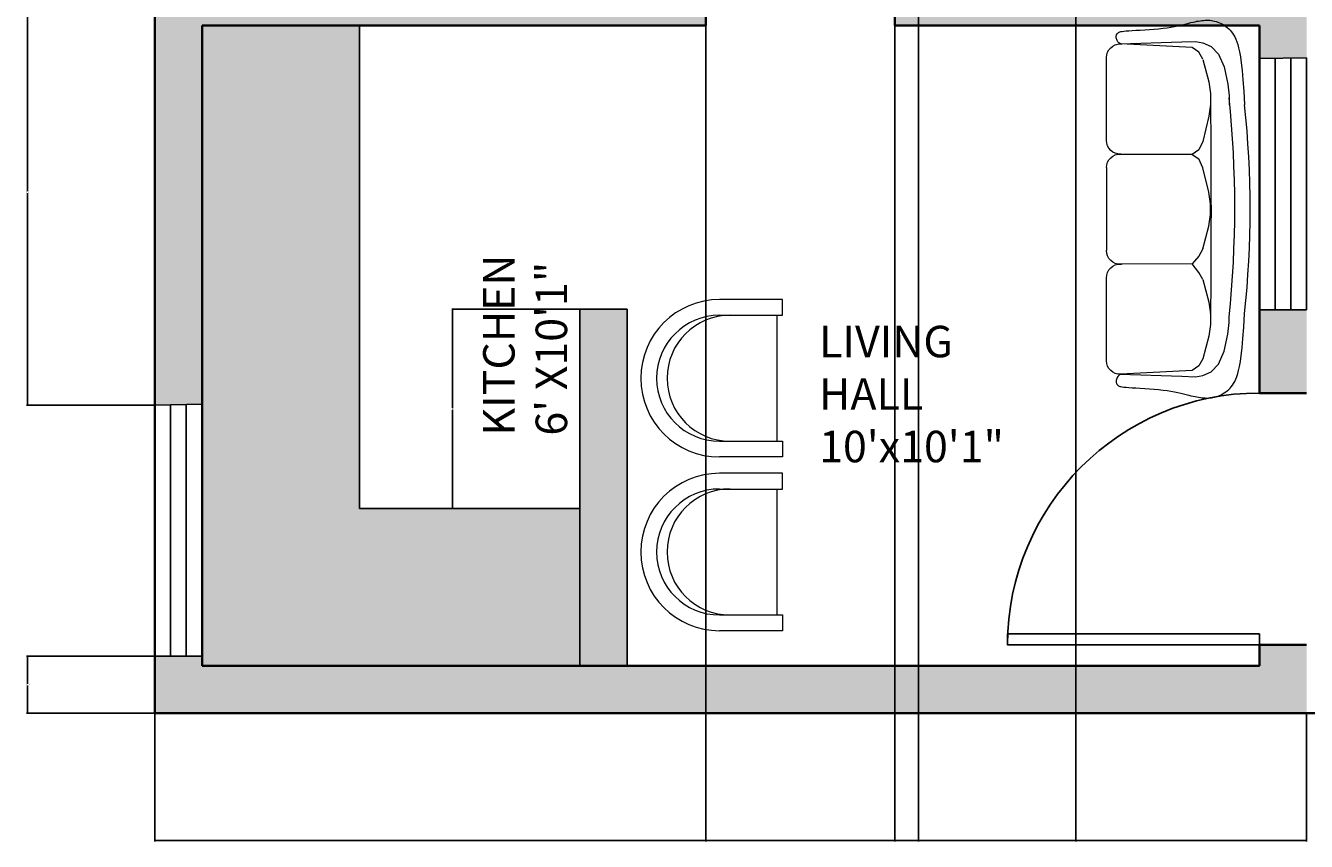
# Model space of a CAD drawing. Units: millimetres. Extents: x 2817 to 5038, y 1110 to 3565.
# Tile 1 of 21: x 2817 to 3061, y 1110 to 1265. Entities that reach past the tile are written whole.
import ezdxf

# ---------------------------------------------------------------- set-up
doc = ezdxf.new("R2010")
doc.units = ezdxf.units.MM
for name, color, linetype, lineweight in [('A-ANNO-DIMS', 2, 'Continuous', 18), ('A-AREA-IDEN', 7, 'Continuous', 18), ('A-FLOR-CASE', 7, 'Continuous', 25), ('A-WALL', 7, 'Continuous', 35), ('DOOR&WINDOW', 1, 'Continuous', 25), ('FURNITURE', 219, 'Continuous', 18)]:
    doc.layers.add(name, color=color, linetype=linetype, lineweight=lineweight)
doc.layers.add('A-FLOR-CASE-PATT', color=251, linetype='Continuous', lineweight=13, true_color=0x636466)
doc.layers.add('A-WALL-PATT', color=51, linetype='Continuous', lineweight=13, true_color=0xf7f281)
doc.styles.get("Standard").update_dxf_attribs({"font": 'arial.ttf'})
doc.dimstyles.get("Standard").update_dxf_attribs({"dimtxt": 0.18, "dimasz": 0.18, "dimexe": 0.18, "dimexo": 0.0625, "dimgap": 0.09, "dimtad": 0, "dimtih": 1, "dimtoh": 1, "dimdec": 4, "dimzin": 0, "dimdsep": 46, "dimtxsty": 'Standard', "dimcen": 0.09, "dimadec": 0, "dimazin": 0, "dimtfac": 1, "dimtdec": 4, "dimtofl": 0, "dimtmove": 0, "dimatfit": 3, "dimfxl": 1, "dimtolj": 1, "dimtzin": 0, "dimarcsym": 0})

# ---------------------------------------------------------------- blocks, each defined once
blk = doc.blocks.new('*U3')
for p, q in [((-40, 0), (-40, 6)), ((0, 0), (0, 6))]:
    blk.add_line(p, q)
blk.add_lwpolyline([(0, 0), (0, -40), (-1.75, -40), (-1.75, 0)], close=True)
blk.add_arc((0, 0), 40, 180, 270)
blk = doc.blocks.new('A$C2E47758B')
for p, q in [((95.4, 1888.9), (87.8, 1883)), ((103.3, 1894.2), (95.4, 1888.9)), ((111.3, 1899.1), (103.3, 1894.2)), ((119.6, 1903.5), (111.3, 1899.1)), ((127.9, 1907.3), (119.6, 1903.5)), ((136.2, 1910.7), (127.9, 1907.3)), ((144.4, 1913.5), (136.2, 1910.7)), ((152.6, 1915.7), (144.4, 1913.5)), ((160.6, 1917.4), (152.6, 1915.7)), ((168.6, 1918.7), (160.6, 1917.4)), ((176.5, 1919.5), (168.6, 1918.7)), ((184.4, 1919.9), (176.5, 1919.5)), ((192.3, 1919.9), (184.4, 1919.9)), ((200.2, 1919.6), (192.3, 1919.9)), ((208.2, 1919.1), (200.2, 1919.6)), ((216.4, 1918.3), (208.2, 1919.1)), ((224.7, 1917.3), (216.4, 1918.3)), ((233.3, 1916), (224.7, 1917.3)), ((242.3, 1914.5), (233.3, 1916)), ((251.8, 1912.6), (242.3, 1914.5)), ((261.8, 1910.5), (251.8, 1912.6)), ((272.6, 1908.1), (261.8, 1910.5)), ((284, 1905.3), (272.6, 1908.1)), ((296.4, 1902.3), (284, 1905.3)), ((309.7, 1899), (296.4, 1902.3)), ((324, 1895.5), (309.7, 1899)), ((339.5, 1892), (324, 1895.5)), ((356.2, 1888.6), (339.5, 1892)), ((374.2, 1885.2), (356.2, 1888.6)), ((44.9, 1823.7), (39.9, 1810.7)), ((50.2, 1835.3), (44.9, 1823.7)), ((55.6, 1845.5), (50.2, 1835.3)), ((61.4, 1854.6), (55.6, 1845.5)), ((67.4, 1862.7), (61.4, 1854.6)), ((73.8, 1870), (67.4, 1862.7)), ((80.6, 1876.8), (73.8, 1870)), ((87.8, 1883), (80.6, 1876.8)), ((393.6, 1882.1), (374.2, 1885.2)), ((414.5, 1879.2), (393.6, 1882.1)), ((436.8, 1876.8), (414.5, 1879.2)), ((460.2, 1874.7), (436.8, 1876.8)), ((484, 1872.9), (460.2, 1874.7)), ((507.6, 1871.3), (484, 1872.9)), ((530.4, 1869.9), (507.6, 1871.3)), ((551.8, 1868.7), (530.4, 1869.9)), ((571.3, 1867.6), (551.8, 1868.7)), ((588.2, 1866.5), (571.3, 1867.6)), ((602.2, 1865.5), (588.2, 1866.5)), ((613.4, 1864.4), (602.2, 1865.5)), ((622.2, 1863.3), (613.4, 1864.4)), ((628.9, 1862.1), (622.2, 1863.3)), ((634, 1860.9), (628.9, 1862.1)), ((637.8, 1859.6), (634, 1860.9)), ((640.6, 1858.2), (637.8, 1859.6)), ((642.9, 1856.7), (640.6, 1858.2)), ((644.9, 1855), (642.9, 1856.7)), ((646.7, 1853.2), (644.9, 1855)), ((648.3, 1851.2), (646.7, 1853.2)), ((649.7, 1849), (648.3, 1851.2)), ((650.8, 1846.6), (649.7, 1849)), ((650, 1821.2), (651.7, 1825.8)), ((651.7, 1843.9), (650.8, 1846.6)), ((652.4, 1840.9), (651.7, 1843.9)), ((651.7, 1825.8), (652.5, 1830.1)), ((652.8, 1837.6), (652.4, 1840.9)), ((652.5, 1830.1), (652.9, 1834)), ((652.9, 1834), (652.8, 1837.6)), ((25.6, 1759.2), (21, 1734.4)), ((30.2, 1779.2), (25.6, 1759.2)), ((35, 1796), (30.2, 1779.2)), ((39.9, 1810.7), (35, 1796)), ((169.1, 1786.1), (133.2, 1748)), ((211.4, 1805.2), (169.1, 1786.1)), ((249.5, 1811.5), (211.4, 1805.2)), ((232.6, 1757.7), (266.4, 1781)), ((232.6, 1757.7), (266.4, 1781)), ((319.3, 1809.4), (249.5, 1811.5)), ((266.4, 1781), (629.3, 1800.3)), ((633, 1799.3), (319.3, 1809.4)), ((626.2, 1798.6), (626.2, 1799)), ((627, 1799), (626.2, 1798.6)), ((633, 1799.3), (639.1, 1805.3)), ((639.1, 1805.3), (643.9, 1810.9)), ((643.9, 1810.9), (647.5, 1816.2)), ((647.5, 1816.2), (650, 1821.2)), ((16.6, 1703.5), (12.3, 1665)), ((21, 1734.4), (16.6, 1703.5)), ((133.2, 1748), (103.5, 1682.4)), ((211.4, 1721.7), (232.6, 1757.7)), ((12.3, 1665), (8.1, 1617.5)), ((103.5, 1682.4), (84.5, 1595.6)), ((8.1, 1617.5), (4, 1559.6)), ((84.5, 1595.6), (78.2, 1536.4)), ((4, 1559.6), (0, 1489.8)), ((78.2, 1536.4), (78.2, 1489.8)), ((78.2, 1515.4), (78.2, 1493.9)), ((211.4, 1169.1), (232.6, 1215)), ((181.8, 1046.7), (211.4, 1169.1)), ((702.1, 1170.7), (702.1, 749.2)), ((173.3, 987.5), (181.8, 1046.7)), ((173.3, 985.3), (173.3, 987.5)), ((173.3, 932.4), (173.3, 985.3)), ((181.8, 873.2), (173.3, 932.4)), ((211.4, 758.9), (181.8, 873.2)), ((211.4, 757.7), (232.6, 721.7)), ((232.6, 721.7), (266.4, 681.7)), ((232.6, 637.5), (266.4, 681.7)), ((266.4, 681.7), (629.3, 680.2)), ((266.4, 681.7), (629.3, 680.2)), ((627, 680.1), (626.2, 679.6)), ((626.2, 679.6), (626.2, 680)), ((627, 679.2), (626.2, 679.6)), ((626.2, 679.6), (626.2, 679.2)), ((211.4, 601.6), (181.8, 487.3)), ((211.4, 601.6), (232.6, 637.5)), ((702.1, 189.8), (702.1, 611.2)), ((181.8, 487.3), (173.3, 428)), ((4, 360.3), (0, 430.1)), ((78.2, 383.5), (78.2, 410.9)), ((173.3, 430.1), (173.3, 373)), ((173.3, 428), (173.3, 430.1)), ((8.1, 302.4), (4, 360.3)), ((84.5, 324.3), (78.2, 383.5)), ((173.3, 373), (181.8, 313.7)), ((12.3, 254.9), (8.1, 302.4)), ((103.5, 237.5), (84.5, 324.3)), ((181.8, 313.7), (211.4, 199.4)), ((16.6, 216.4), (12.3, 254.9)), ((21, 185.5), (16.6, 216.4)), ((133.2, 171.9), (103.5, 237.5)), ((211.4, 199.4), (232.6, 163.4)), ((25.6, 160.7), (21, 185.5)), ((30.2, 140.7), (25.6, 160.7)), ((35, 123.9), (30.2, 140.7)), ((169.1, 133.8), (133.2, 171.9)), ((211.4, 114.7), (169.1, 133.8)), ((232.6, 163.4), (266.4, 140.1)), ((266.4, 140.1), (629.3, 120.7)), ((39.9, 109.2), (35, 123.9)), ((44.9, 96.2), (39.9, 109.2)), ((50.2, 84.6), (44.9, 96.2)), ((55.6, 74.4), (50.2, 84.6)), ((61.4, 65.3), (55.6, 74.4)), ((67.4, 57.2), (61.4, 65.3)), ((249.5, 108.4), (211.4, 114.7)), ((319.3, 110.5), (249.5, 108.4)), ((633, 120.7), (319.3, 110.5)), ((626.2, 121.3), (626.2, 120.9)), ((627, 120.9), (626.2, 121.3)), ((633, 120.7), (639.1, 114.6)), ((639.1, 114.6), (643.9, 109)), ((643.9, 109), (647.5, 103.7)), ((646.7, 66.7), (644.9, 64.9)), ((648.3, 68.7), (646.7, 66.7)), ((647.5, 103.7), (650, 98.7)), ((649.7, 70.9), (648.3, 68.7)), ((650.8, 73.3), (649.7, 70.9)), ((650, 98.7), (651.7, 94.1)), ((651.7, 76), (650.8, 73.3)), ((651.7, 94.1), (652.5, 89.8)), ((652.4, 79), (651.7, 76)), ((652.8, 82.3), (652.4, 79)), ((652.5, 89.8), (652.9, 85.9)), ((652.9, 85.9), (652.8, 82.3)), ((73.8, 49.9), (67.4, 57.2)), ((80.6, 43.1), (73.8, 49.9)), ((87.8, 36.9), (80.6, 43.1)), ((95.4, 31.1), (87.8, 36.9)), ((103.3, 25.7), (95.4, 31.1)), ((111.3, 20.8), (103.3, 25.7)), ((119.6, 16.4), (111.3, 20.8)), ((127.9, 12.6), (119.6, 16.4)), ((136.2, 9.2), (127.9, 12.6)), ((144.4, 6.4), (136.2, 9.2)), ((152.6, 4.2), (144.4, 6.4)), ((160.6, 2.5), (152.6, 4.2)), ((168.6, 1.3), (160.6, 2.5)), ((176.5, 0.5), (168.6, 1.3)), ((184.4, 0), (176.5, 0.5)), ((192.3, 0), (184.4, 0)), ((200.2, 0.3), (192.3, 0)), ((208.2, 0.8), (200.2, 0.3)), ((216.4, 1.6), (208.2, 0.8)), ((224.7, 2.6), (216.4, 1.6)), ((233.3, 3.9), (224.7, 2.6)), ((242.3, 5.4), (233.3, 3.9)), ((251.8, 7.3), (242.3, 5.4)), ((261.8, 9.4), (251.8, 7.3)), ((272.6, 11.8), (261.8, 9.4)), ((284, 14.6), (272.6, 11.8)), ((296.4, 17.6), (284, 14.6)), ((309.7, 20.9), (296.4, 17.6)), ((324, 24.4), (309.7, 20.9)), ((339.5, 27.9), (324, 24.4)), ((356.2, 31.4), (339.5, 27.9)), ((374.2, 34.7), (356.2, 31.4)), ((393.6, 37.8), (374.2, 34.7)), ((414.5, 40.7), (393.6, 37.8)), ((436.8, 43.1), (414.5, 40.7)), ((460.2, 45.2), (436.8, 43.1)), ((484, 47), (460.2, 45.2)), ((507.6, 48.6), (484, 47)), ((530.4, 50), (507.6, 48.6)), ((551.8, 51.2), (530.4, 50)), ((571.3, 52.3), (551.8, 51.2)), ((588.2, 53.4), (571.3, 52.3)), ((602.2, 54.4), (588.2, 53.4)), ((613.4, 55.5), (602.2, 54.4)), ((622.2, 56.6), (613.4, 55.5)), ((628.9, 57.8), (622.2, 56.6)), ((634, 59), (628.9, 57.8)), ((637.8, 60.3), (634, 59)), ((640.6, 61.7), (637.8, 60.3)), ((642.9, 63.2), (640.6, 61.7)), ((644.9, 64.9), (642.9, 63.2))]:
    blk.add_line(p, q)
for points in [[(629.3, 1239.7), (266.4, 1238.2), (629.3, 1239.7, 0.429937), (702.1, 1308.7), (702.1, 1730.1, 0.429937), (629.3, 1799.2)], [(78.2, 410.9, -0.050936), (78.2, 1525.6, 12.167348)], [(0, 430.1, -0.05358), (0, 1489.8, 12.163767)], [(173.3, 1494, 0.004989), (173.3, 401.5, 0.847003)]]:
    blk.add_lwpolyline(points, format="xyb")
blk.add_lwpolyline([(211.4, 1720.5), (181.8, 1606.2), (173.3, 1546.9), (173.3, 1494), (173.3, 1491.9), (181.8, 1432.6), (211.4, 1304.3), (232.6, 1261.5), (266.4, 1238.2), (232.6, 1215)])
for centre, start, end in [((633, 1170.7), 0, 93.05866), ((633, 749.2), 266.94134, 360), ((633, 749.2), 266.94134, 360), ((633, 611.2), 0, 93.05866), ((633, 611.2), 0, 93.05866), ((633, 611.2), 0, 93.05866), ((633, 189.8), 266.94134, 360)]:
    blk.add_arc(centre, 69.1, start, end)
blk = doc.blocks.new('12PSTG07')
at = {"color": 0, "linetype": 'ByBlock'}
for p, q in [((0, 15), (-12, 15)), ((0, 12), (0, 15)), ((-12, 12), (0, 12)), ((-1, -12), (-1, 12)), ((-12, -12), (0, -12)), ((0, -12), (0, -15)), ((0, -15), (-12, -15))]:
    blk.add_line(p, q, dxfattribs=at)
for centre, radius in [((-12, 0), 15), ((-12, 0), 12), ((-10, 0), 12)]:
    blk.add_arc(centre, radius, 90, 270, dxfattribs=at)
blk = doc.blocks.new('WIN-4FT')
for p, q in [((0, 47.85), (9, 48)), ((0, 0), (0, 47.85)), ((3, 0), (3, 47.85)), ((6, 48), (6, 0)), ((9, 48), (9, 0)), ((9, 0), (0, 0))]:
    blk.add_line(p, q)
blk = doc.blocks.new('*D28')
at = {"layer": 'A-ANNO-DIMS', "color": 0, "lineweight": -2, "transparency": 16777216}
for p, q in [((2841.74, 1134.37), (2841.74, 1110.01)), ((3061.24, 1134.37), (3061.24, 1110.01)), ((2841.92, 1110.19), (2951.09, 1110.19)), ((3061.06, 1110.19), (2951.89, 1110.19))]:
    blk.add_line(p, q, dxfattribs=at)
for points in [[(2841.92, 1110.22), (2841.92, 1110.16), (2841.74, 1110.19)], [(3061.06, 1110.22), (3061.06, 1110.16), (3061.24, 1110.19)]]:
    blk.add_solid(points, dxfattribs=at)
at = {"layer": 'Defpoints', "color": 0, "lineweight": -2, "transparency": 16777216}
for p in [(2841.74, 1134.44), (3061.24, 1134.44), (3061.24, 1110.19)]:
    blk.add_point(p, dxfattribs=at)
at = {"layer": 'A-ANNO-DIMS', "color": 0, "transparency": 16777216, "insert": (2951.49, 1110.19), "char_height": 0.18, "attachment_point": 5}
blk.add_mtext('\\A1;219.5', dxfattribs=at)
blk = doc.blocks.new('*D30')
at = {"layer": 'A-ANNO-DIMS', "color": 0, "lineweight": -2, "transparency": 16777216}
for p, q in [((2841.68, 1145.3), (2817.31, 1145.3)), ((2817.49, 1145.12), (2817.49, 1140.05)), ((2817.49, 1134.62), (2817.49, 1139.69)), ((2841.68, 1134.44), (2817.31, 1134.44))]:
    blk.add_line(p, q, dxfattribs=at)
for points in [[(2817.46, 1145.12), (2817.52, 1145.12), (2817.49, 1145.3)], [(2817.46, 1134.62), (2817.52, 1134.62), (2817.49, 1134.44)]]:
    blk.add_solid(points, dxfattribs=at)
at = {"layer": 'Defpoints', "color": 0, "lineweight": -2, "transparency": 16777216}
for p in [(2817.49, 1145.3), (2841.74, 1145.3), (2841.74, 1134.44)]:
    blk.add_point(p, dxfattribs=at)
at = {"layer": 'A-ANNO-DIMS', "color": 0, "transparency": 16777216, "insert": (2817.49, 1139.87), "char_height": 0.18, "attachment_point": 5}
blk.add_mtext('\\A1;10.864', dxfattribs=at)
blk = doc.blocks.new('*D31')
at = {"layer": 'A-ANNO-DIMS', "color": 0, "lineweight": -2, "transparency": 16777216}
for p, q in [((2841.68, 1274.26), (2817.31, 1274.26)), ((2817.49, 1274.08), (2817.49, 1233.89)), ((2817.49, 1193.33), (2817.49, 1233.52)), ((2841.68, 1193.15), (2817.31, 1193.15))]:
    blk.add_line(p, q, dxfattribs=at)
for points in [[(2817.46, 1274.08), (2817.52, 1274.08), (2817.49, 1274.26)], [(2817.46, 1193.33), (2817.52, 1193.33), (2817.49, 1193.15)]]:
    blk.add_solid(points, dxfattribs=at)
at = {"layer": 'Defpoints', "color": 0, "lineweight": -2, "transparency": 16777216}
for p in [(2817.49, 1274.26), (2841.74, 1274.26), (2841.74, 1193.15)]:
    blk.add_point(p, dxfattribs=at)
at = {"layer": 'A-ANNO-DIMS', "color": 0, "transparency": 16777216, "insert": (2817.49, 1233.7), "char_height": 0.18, "attachment_point": 5}
blk.add_mtext('\\A1;81.1', dxfattribs=at)
blk = doc.blocks.new('*D34')
at = {"layer": 'A-ANNO-DIMS', "color": 0, "lineweight": -2, "transparency": 16777216}
for p, q in [((2946.74, 1500.37), (2946.74, 1110.01)), ((2982.74, 1500.37), (2982.74, 1110.01)), ((2946.92, 1110.19), (2964.52, 1110.19)), ((2982.56, 1110.19), (2964.96, 1110.19))]:
    blk.add_line(p, q, dxfattribs=at)
for points in [[(2946.92, 1110.22), (2946.92, 1110.16), (2946.74, 1110.19)], [(2982.56, 1110.22), (2982.56, 1110.16), (2982.74, 1110.19)]]:
    blk.add_solid(points, dxfattribs=at)
at = {"layer": 'Defpoints', "color": 0, "lineweight": -2, "transparency": 16777216}
for p in [(2946.74, 1500.44), (2982.74, 1500.44), (2982.74, 1110.19)]:
    blk.add_point(p, dxfattribs=at)
at = {"layer": 'A-ANNO-DIMS', "color": 0, "transparency": 16777216, "insert": (2964.74, 1110.19), "char_height": 0.18, "attachment_point": 5}
blk.add_mtext('\\A1;36', dxfattribs=at)
blk = doc.blocks.new('*D35')
at = {"layer": 'A-ANNO-DIMS', "color": 0, "lineweight": -2, "transparency": 16777216}
for p, q in [((2987.24, 1605.37), (2987.24, 1110.01)), ((3017.24, 1605.37), (3017.24, 1110.01)), ((2987.42, 1110.19), (3002.02, 1110.19)), ((3017.06, 1110.19), (3002.46, 1110.19))]:
    blk.add_line(p, q, dxfattribs=at)
for points in [[(2987.42, 1110.22), (2987.42, 1110.16), (2987.24, 1110.19)], [(3017.06, 1110.22), (3017.06, 1110.16), (3017.24, 1110.19)]]:
    blk.add_solid(points, dxfattribs=at)
at = {"layer": 'Defpoints', "color": 0, "lineweight": -2, "transparency": 16777216}
for p in [(2987.24, 1605.44), (3017.24, 1605.44), (3017.24, 1110.19)]:
    blk.add_point(p, dxfattribs=at)
at = {"layer": 'A-ANNO-DIMS', "color": 0, "transparency": 16777216, "insert": (3002.24, 1110.19), "char_height": 0.18, "attachment_point": 5}
blk.add_mtext('\\A1;30', dxfattribs=at)
blk = doc.blocks.new('*D45')
at = {"layer": 'A-ANNO-DIMS', "color": 0, "lineweight": -2, "transparency": 16777216}
for p, q in [((2922.68, 1211.44), (2898.31, 1211.44)), ((2898.49, 1211.26), (2898.49, 1192.62)), ((2898.49, 1173.62), (2898.49, 1192.25)), ((2922.68, 1173.44), (2898.31, 1173.44))]:
    blk.add_line(p, q, dxfattribs=at)
for points in [[(2898.46, 1211.26), (2898.52, 1211.26), (2898.49, 1211.44)], [(2898.46, 1173.62), (2898.52, 1173.62), (2898.49, 1173.44)]]:
    blk.add_solid(points, dxfattribs=at)
at = {"layer": 'Defpoints', "color": 0, "lineweight": -2, "transparency": 16777216}
for p in [(2898.49, 1211.44), (2922.74, 1211.44), (2922.74, 1173.44)]:
    blk.add_point(p, dxfattribs=at)
at = {"layer": 'A-ANNO-DIMS', "color": 0, "transparency": 16777216, "insert": (2898.49, 1192.44), "char_height": 0.18, "attachment_point": 5}
blk.add_mtext('\\A1;38', dxfattribs=at)

msp = doc.modelspace()

# ---------------------------------------------------------------- hatches: boundary and pattern name
at = {"layer": 'A-FLOR-CASE-PATT'}
h = msp.add_hatch(color=256, dxfattribs=at)
h.dxf.hatch_style = 1
h.paths.add_polyline_path([(2931.7393, 1458.4357), (2922.7393, 1458.4357), (2922.7393, 1379.4357), (2931.7393, 1379.4357)])
h.paths.add_polyline_path([(2931.7393, 1211.4357), (2922.7393, 1211.4357), (2922.7393, 1143.4357), (2931.7393, 1143.4357)])
h = msp.add_hatch(color=256, dxfattribs=at)
h.dxf.hatch_style = 1
h.paths.add_polyline_path([(2931.7393, 1458.4357), (2922.7393, 1458.4357), (2922.7393, 1379.4357), (2931.7393, 1379.4357)])
h.paths.add_polyline_path([(2931.7393, 1211.4357), (2922.7393, 1211.4357), (2922.7393, 1143.4357), (2931.7393, 1143.4357)])
h = msp.add_hatch(color=256, dxfattribs=at)
h.dxf.hatch_style = 1
h.paths.add_polyline_path([(2922.7393, 1173.4357), (2880.7393, 1173.4357), (2880.7393, 1265.4357), (2850.7393, 1265.4357), (2850.7393, 1143.4357), (2922.7393, 1143.4357)])
at = {"layer": 'A-WALL-PATT'}
h = msp.add_hatch(color=256, dxfattribs=at)
h.dxf.hatch_style = 1
h.paths.add_polyline_path([(3186.7393, 1614.4357), (2841.7393, 1614.4357), (2841.7393, 1568.614), (2850.7393, 1568.7609), (2850.7393, 1605.4357), (2982.7393, 1605.4357), (2991.7393, 1605.4357), (3052.2393, 1605.4357), (3052.2393, 1573.7835), (3061.2393, 1573.7835), (3061.2393, 1605.4357), (3182.2393, 1605.4357), (3182.2393, 1143.4357), (3181.2393, 1143.4357), (3181.2393, 1134.4357), (3186.7393, 1134.4357)])
h.paths.add_polyline_path([(3061.2393, 1143.4357), (3061.2393, 1147.4357), (3052.2393, 1147.4357), (3052.2393, 1143.4357), (2850.7393, 1143.4357), (2850.7393, 1145.2996), (2841.7393, 1145.2996), (2841.7393, 1134.4357), (3061.2393, 1134.4357)], flags=17)
h.paths.add_polyline_path([(2850.7393, 1265.4357), (2946.7393, 1265.4357), (2946.7393, 1270.8357), (2946.7393, 1274.4357), (2850.7393, 1274.4357), (2850.7381, 1274.4357), (2850.7381, 1274.2564), (2841.7393, 1274.2564), (2841.7393, 1193.1527), (2850.7393, 1193.2996)], flags=17)
h.paths.add_polyline_path([(3061.2393, 1299.098), (3052.2393, 1299.098), (3052.2393, 1274.4357), (2991.7393, 1274.4357), (2991.7393, 1340.4357), (2982.7393, 1340.4357), (2982.7393, 1274.4357), (2982.7393, 1265.4357), (3052.2393, 1265.4357), (3052.2393, 1259.143), (3061.2393, 1259.2899)], flags=17)
h.paths.add_polyline_path([(3061.2393, 1383.4357), (3052.2393, 1383.4357), (3052.2393, 1379.4357), (2931.7393, 1379.4357), (2922.7393, 1379.4357), (2850.7393, 1379.4357), (2850.7381, 1379.4357), (2850.7381, 1379.3646), (2841.7393, 1379.3646), (2841.7393, 1322.1095), (2850.7393, 1322.2564), (2850.7393, 1370.4357), (2982.7393, 1370.4357), (2987.2393, 1370.4357), (3017.2393, 1370.4357), (3052.2393, 1370.4357), (3052.2393, 1323.098), (3061.2393, 1323.098)], flags=17)
h = msp.add_hatch(color=256, dxfattribs=at)
h.dxf.hatch_style = 1
h.paths.add_polyline_path([(3061.2393, 1549.7835), (3052.2393, 1549.7835), (3052.2393, 1509.4357), (2991.7393, 1509.4357), (2991.7393, 1575.4357), (2982.7393, 1575.4357), (2982.7393, 1509.4357), (2982.7393, 1500.4357), (3052.2393, 1500.4357), (3052.2393, 1498.4661), (3061.2393, 1498.613)])
h.paths.add_polyline_path([(2946.7393, 1505.8357), (2946.7393, 1509.4357), (2850.7393, 1509.4357), (2850.7393, 1520.7609), (2841.7393, 1520.7609), (2841.7393, 1427.2177), (2850.7393, 1427.3646), (2850.7393, 1500.4357), (2922.7393, 1500.4357), (2931.7393, 1500.4357), (2946.7393, 1500.4357)])
h.paths.add_polyline_path([(3061.2393, 1450.613), (3052.2393, 1450.613), (3052.2393, 1431.4357), (3059.4393, 1431.4357), (3061.2393, 1431.4357)])
h.paths.add_polyline_path([(3061.2393, 1211.2899), (3052.2393, 1211.2899), (3052.2393, 1195.4357), (3059.4393, 1195.4357), (3061.2393, 1195.4357)])

# ---------------------------------------------------------------- linework, layer by layer
at = {"layer": 'A-FLOR-CASE'}
for p, q in [((2880.7393, 1173.4357), (2880.7393, 1265.4357)), ((2922.7393, 1143.4357), (2922.7393, 1211.4357)), ((2922.7393, 1211.4357), (2931.7393, 1211.4357)), ((2931.7393, 1143.4357), (2931.7393, 1211.4357)), ((2922.7393, 1173.4357), (2880.7393, 1173.4357))]:
    msp.add_line(p, q, dxfattribs=at)
at = {"layer": 'A-WALL'}
for p, q in [((2841.7393, 1134.4357), (2841.7393, 1614.4357)), ((2946.7393, 1274.4357), (2946.7393, 1265.4357)), ((2982.7393, 1274.4357), (2982.7393, 1265.4357)), ((2850.7393, 1143.4357), (2850.7393, 1265.4357)), ((2850.7393, 1265.4357), (2946.7393, 1265.4357)), ((2982.7393, 1265.4357), (3052.2393, 1265.4357)), ((3052.2393, 1265.4357), (3052.2393, 1195.4357)), ((3052.2393, 1195.4357), (3061.2393, 1195.4357)), ((3052.2393, 1147.4357), (3061.2393, 1147.4357)), ((3052.2393, 1147.4357), (3052.2393, 1143.4357)), ((3052.2393, 1143.4357), (2850.7393, 1143.4357)), ((3186.7393, 1134.4357), (2841.7393, 1134.4357))]:
    msp.add_line(p, q, dxfattribs=at)

# ---------------------------------------------------------------- block references
at = {"layer": 'DOOR&WINDOW'}
for p in [(3052.2393, 1211.2898), (2841.7393, 1145.2995)]:
    msp.add_blockref('WIN-4FT', p, dxfattribs=at)
at = {"layer": 'DOOR&WINDOW', "xscale": 1.199999999999999, "yscale": 1.199999999999999, "zscale": 1.199999999999999, "rotation": 270}
msp.add_blockref('*U3', (3052.2393, 1147.4357), dxfattribs=at)
at = {"layer": 'FURNITURE', "xscale": -0.0374923371980192, "yscale": 0.0374923371980192, "zscale": 0.0374923371980192}
msp.add_blockref('A$C2E47758B', (3049.4066, 1194.48), dxfattribs=at)
at = {"layer": 'FURNITURE'}
for p in [(2961.3521, 1198.2437), (2961.3521, 1165.1449)]:
    msp.add_blockref('12PSTG07', p, dxfattribs=at)

# ---------------------------------------------------------------- texts
at = {"layer": 'A-AREA-IDEN', "insert": (2904.303, 1187.3161), "char_height": 6, "attachment_point": 1, "rotation": 90}
msp.add_mtext_dynamic_manual_height_columns('KITCHEN\\P6\' X10\'1"', width=42.068425, gutter_width=12.5, heights=[0], dxfattribs=at)
at = {"layer": 'A-AREA-IDEN', "insert": (2968.3328, 1208.2403), "char_height": 6, "attachment_point": 1}
msp.add_mtext_dynamic_manual_height_columns('LIVING HALL\\P10\'x10\'1"', width=42.068425, gutter_width=12.5, heights=[0], dxfattribs=at)

# ---------------------------------------------------------------- dimensions: what is measured, and where the dimension line sits
at = {"layer": 'A-ANNO-DIMS'}
for base, p1, p2, override, picture, middle in [((3017.2393, 1110.1857), (2987.2393, 1605.4357), (3017.2393, 1605.4357), {"dimdec": 0, "dimlfac": 1, "dimrnd": 0, "dimzin": 0, "dimdsep": 46, "dimlunit": 2}, '*D35', (3002.2393, 1110.1857)), ((2982.7393, 1110.1857), (2946.7393, 1500.4357), (2982.7393, 1500.4357), {"dimdec": 0, "dimlfac": 1, "dimrnd": 0, "dimzin": 0, "dimdsep": 46, "dimlunit": 2}, '*D34', (2964.7393, 1110.1857)), ((3061.2393, 1110.1857), (2841.7393, 1134.4357), (3061.2393, 1134.4357), {"dimdec": 1, "dimlfac": 1, "dimrnd": 0, "dimzin": 0, "dimdsep": 46, "dimlunit": 2}, '*D28', (2951.4893, 1110.1857))]:
    dim = msp.add_linear_dim(base=base, p1=p1, p2=p2, dimstyle='Standard', override=override, dxfattribs=at)
    dim.commit()
    dim.dimension.update_dxf_attribs({"geometry": picture, "text_midpoint": middle})
for base, p1, p2, override, picture, middle in [((2817.4881, 1274.2564), (2841.7405, 1193.1527), (2841.7381, 1274.2564), {"dimdec": 1, "dimlfac": 1, "dimrnd": 0, "dimzin": 0, "dimdsep": 46, "dimlunit": 2}, '*D31', (2817.4881, 1233.7046)), ((2898.4893, 1211.4357), (2922.7393, 1173.4357), (2922.7393, 1211.4357), {"dimdec": 0, "dimlfac": 1, "dimrnd": 0, "dimzin": 0, "dimdsep": 46, "dimlunit": 2}, '*D45', (2898.4893, 1192.4357)), ((2817.4881, 1145.2996), (2841.7393, 1134.4357), (2841.7393, 1145.2996), {"dimdec": 3, "dimlfac": 1, "dimrnd": 0, "dimzin": 0, "dimdsep": 46, "dimlunit": 2}, '*D30', (2817.4881, 1139.8676))]:
    dim = msp.add_linear_dim(base=base, p1=p1, p2=p2, angle=90, dimstyle='Standard', override=override, dxfattribs=at)
    dim.commit()
    dim.dimension.update_dxf_attribs({"geometry": picture, "text_midpoint": middle})

doc.saveas('drawing.dxf')
